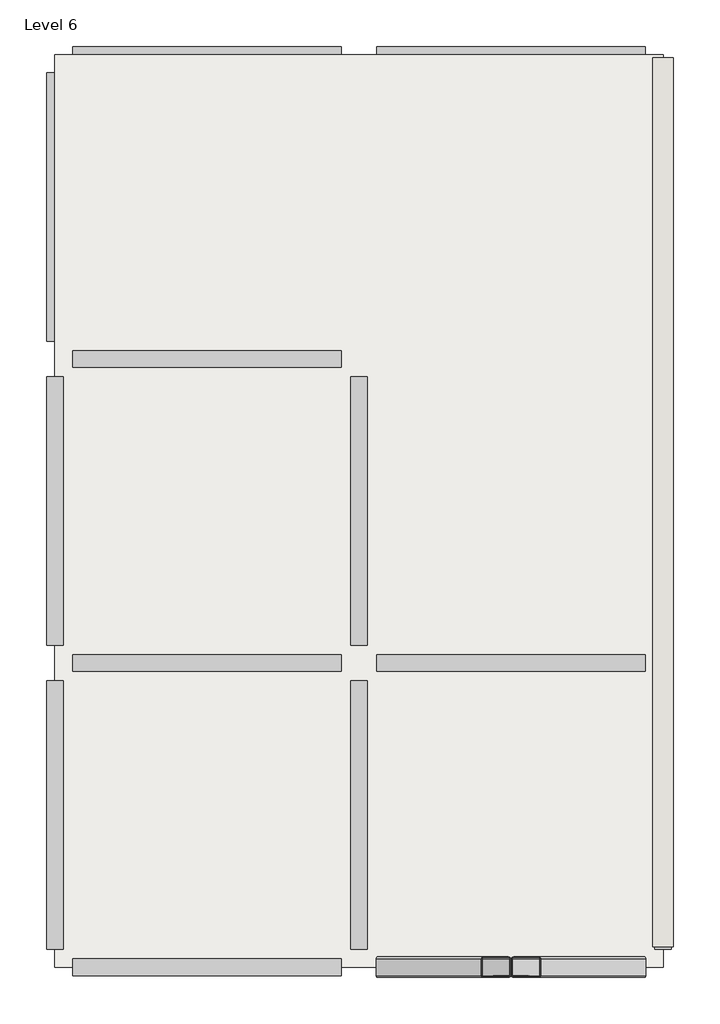
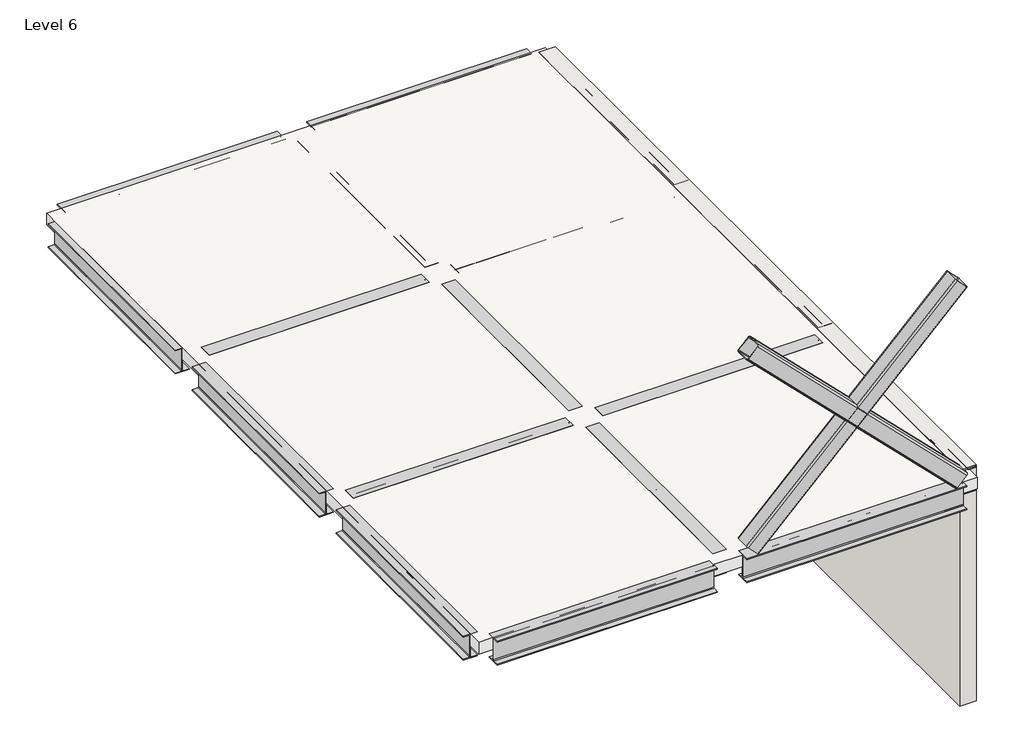
# One storey: 17 beams, 2 members, 1 slab, 1 wall.
"""IFC4 building model written with IfcOpenShell, lengths in millimetres."""

from ifc_helpers import new_model, si_unit, frame, origin, place, context, project, spatial, polyline, outline, extrude, transform, mapped, element, save
from components import ub_universal_beams_ub305x165x40_60ab2ee1, m_hss_square_hss203_2x203_2x9_5_07d005dd

model = new_model("IFC4")

# Units and contexts
model_context = context("Model", 3, world=origin())
ifc_project = project(units=[si_unit("LENGTHUNIT", "METRE", prefix="MILLI")], contexts=[model_context])

# Site, building, storey
site = spatial("IfcSite", under=ifc_project)
building = spatial("IfcBuilding", under=site)
storey = spatial("IfcBuildingStorey", under=building, Name="Level 6", Elevation=15000.0)

# Beams
placement = place(None, origin())
ub_universal_beams_ub305x165x40_shape = ub_universal_beams_ub305x165x40_60ab2ee1(model_context)
element("IfcBeam", 1, ObjectType="UB-Universal Beams : UB305x165x40", at=placement, inside=storey, context=model_context, shape_type="MappedRepresentation", body=[
    mapped(ub_universal_beams_ub305x165x40_shape, transform((18435.1404262, -6314.7314166, 14848.3), x_axis=(-1.0, 0.0, 0.0), y_axis=(0.0, -1.0, 0.0), z_axis=(0.0, 0.0, 1.0))),
])
element("IfcBeam", 2, ObjectType="UB-Universal Beams : UB305x165x40", at=placement, inside=storey, context=model_context, shape_type="MappedRepresentation", body=[
    mapped(ub_universal_beams_ub305x165x40_shape, transform((15435.1404262, -6314.7314166, 14848.3), x_axis=(-1.0, 0.0, 0.0), y_axis=(0.0, -1.0, 0.0), z_axis=(0.0, 0.0, 1.0))),
])
element("IfcBeam", 3, ObjectType="UB-Universal Beams : UB305x165x40", at=placement, inside=storey, context=model_context, shape_type="MappedRepresentation", body=[
    mapped(ub_universal_beams_ub305x165x40_shape, transform((13935.1404262, -4814.7314166, 14848.3), x_axis=(0.0, 1.0, 0.0), y_axis=(-1.0, 0.0, 0.0), z_axis=(0.0, 0.0, 1.0))),
])
element("IfcBeam", 4, ObjectType="UB-Universal Beams : UB305x165x40", at=placement, inside=storey, context=model_context, shape_type="MappedRepresentation", body=[
    mapped(ub_universal_beams_ub305x165x40_shape, transform((13935.1404262, -1814.7314166, 14848.3), x_axis=(0.0, 1.0, 0.0), y_axis=(-1.0, 0.0, 0.0), z_axis=(0.0, 0.0, 1.0))),
])
element("IfcBeam", 5, ObjectType="UB-Universal Beams : UB305x165x40", at=placement, inside=storey, context=model_context, shape_type="MappedRepresentation", body=[
    mapped(ub_universal_beams_ub305x165x40_shape, transform((13935.1404262, 1185.2685834, 14848.3), x_axis=(0.0, 1.0, 0.0), y_axis=(-1.0, 0.0, 0.0), z_axis=(0.0, 0.0, 1.0))),
])
element("IfcBeam", 6, ObjectType="UB-Universal Beams : UB305x165x40", at=placement, inside=storey, context=model_context, shape_type="MappedRepresentation", body=[
    mapped(ub_universal_beams_ub305x165x40_shape, transform((18435.1404262, -3314.7314166, 14848.3), x_axis=(-1.0, 0.0, 0.0), y_axis=(0.0, -1.0, 0.0), z_axis=(0.0, 0.0, 1.0))),
])
element("IfcBeam", 7, ObjectType="UB-Universal Beams : UB305x165x40", at=placement, inside=storey, context=model_context, shape_type="MappedRepresentation", body=[
    mapped(ub_universal_beams_ub305x165x40_shape, transform((15435.1404262, -3314.7314166, 14848.3), x_axis=(-1.0, 0.0, 0.0), y_axis=(0.0, -1.0, 0.0), z_axis=(0.0, 0.0, 1.0))),
])
element("IfcBeam", 8, ObjectType="UB-Universal Beams : UB305x165x40", at=placement, inside=storey, context=model_context, shape_type="MappedRepresentation", body=[
    mapped(ub_universal_beams_ub305x165x40_shape, transform((18435.1404262, -314.7314166, 14848.3), x_axis=(-1.0, 0.0, 0.0), y_axis=(0.0, -1.0, 0.0), z_axis=(0.0, 0.0, 1.0))),
])
element("IfcBeam", 9, ObjectType="UB-Universal Beams : UB305x165x40", at=placement, inside=storey, context=model_context, shape_type="MappedRepresentation", body=[
    mapped(ub_universal_beams_ub305x165x40_shape, transform((15435.1404262, -314.7314166, 14848.3), x_axis=(-1.0, 0.0, 0.0), y_axis=(0.0, -1.0, 0.0), z_axis=(0.0, 0.0, 1.0))),
])
element("IfcBeam", 10, ObjectType="UB-Universal Beams : UB305x165x40", at=placement, inside=storey, context=model_context, shape_type="MappedRepresentation", body=[
    mapped(ub_universal_beams_ub305x165x40_shape, transform((18435.1404262, 2685.2685834, 14848.3), x_axis=(-1.0, 0.0, 0.0), y_axis=(0.0, -1.0, 0.0), z_axis=(0.0, 0.0, 1.0))),
])
element("IfcBeam", 11, ObjectType="UB-Universal Beams : UB305x165x40", at=placement, inside=storey, context=model_context, shape_type="MappedRepresentation", body=[
    mapped(ub_universal_beams_ub305x165x40_shape, transform((15435.1404262, 2685.2685834, 14848.3), x_axis=(-1.0, 0.0, 0.0), y_axis=(0.0, -1.0, 0.0), z_axis=(0.0, 0.0, 1.0))),
])
element("IfcBeam", 12, ObjectType="UB-Universal Beams : UB305x165x40", at=placement, inside=storey, context=model_context, shape_type="MappedRepresentation", body=[
    mapped(ub_universal_beams_ub305x165x40_shape, transform((16935.1404262, -4814.7314166, 14848.3), x_axis=(0.0, 1.0, 0.0), y_axis=(-1.0, 0.0, 0.0), z_axis=(0.0, 0.0, 1.0))),
])
element("IfcBeam", 13, ObjectType="UB-Universal Beams : UB305x165x40", at=placement, inside=storey, context=model_context, shape_type="MappedRepresentation", body=[
    mapped(ub_universal_beams_ub305x165x40_shape, transform((16935.1404262, -1814.7314166, 14848.3), x_axis=(0.0, 1.0, 0.0), y_axis=(-1.0, 0.0, 0.0), z_axis=(0.0, 0.0, 1.0))),
])
element("IfcBeam", 14, ObjectType="UB-Universal Beams : UB305x165x40", at=placement, inside=storey, context=model_context, shape_type="MappedRepresentation", body=[
    mapped(ub_universal_beams_ub305x165x40_shape, transform((16935.1404262, 1185.2685834, 14848.3), x_axis=(0.0, 1.0, 0.0), y_axis=(-1.0, 0.0, 0.0), z_axis=(0.0, 0.0, 1.0))),
])
element("IfcBeam", 15, ObjectType="UB-Universal Beams : UB305x165x40", at=placement, inside=storey, context=model_context, shape_type="MappedRepresentation", body=[
    mapped(ub_universal_beams_ub305x165x40_shape, transform((19935.1404262, -1814.7314166, 14848.3), x_axis=(0.0, 1.0, 0.0), y_axis=(-1.0, 0.0, 0.0), z_axis=(0.0, 0.0, 1.0))),
])
element("IfcBeam", 16, ObjectType="UB-Universal Beams : UB305x165x40", at=placement, inside=storey, context=model_context, shape_type="MappedRepresentation", body=[
    mapped(ub_universal_beams_ub305x165x40_shape, transform((19935.1404262, 1185.2685834, 14848.3), x_axis=(0.0, 1.0, 0.0), y_axis=(-1.0, 0.0, 0.0), z_axis=(0.0, 0.0, 1.0))),
])
element("IfcBeam", 17, ObjectType="UB-Universal Beams : beam", at=placement, inside=storey, context=model_context, shape_type="MappedRepresentation", body=[
    mapped(ub_universal_beams_ub305x165x40_shape, transform((19935.1404262, -4814.7314166, 14848.3), x_axis=(0.0, 1.0, 0.0), y_axis=(-1.0, 0.0, 0.0), z_axis=(0.0, 0.0, 1.0))),
])

# Members
m_hss_square_hss203_2x203_2x9_5_shape = m_hss_square_hss203_2x203_2x9_5_07d005dd(model_context)
element("IfcMember", 18, ObjectType="M_HSS Square : HSS203.2X203.2X9.5", at=placement, inside=storey, context=model_context, shape_type="MappedRepresentation", body=[
    mapped(m_hss_square_hss203_2x203_2x9_5_shape, transform((18435.1404262, -6314.7314166, 16348.3), x_axis=(-0.7071067811865478, 0.0, 0.7071067811865476), y_axis=(0.0, -1.0000000000000002, 0.0), z_axis=(0.7071067811865476, 0.0, 0.7071067811865478))),
])
element("IfcMember", 19, ObjectType="M_HSS Square : HSS203.2X203.2X9.5", at=placement, inside=storey, context=model_context, shape_type="MappedRepresentation", body=[
    mapped(m_hss_square_hss203_2x203_2x9_5_shape, transform((18435.1404262, -6314.7314166, 16348.3), x_axis=(-0.7071067811865478, 0.0, -0.7071067811865475), y_axis=(0.0, -1.0000000000000002, 0.0), z_axis=(-0.7071067811865475, 0.0, 0.7071067811865478))),
])

# Slab
element("IfcSlab", 20, ObjectType="150mm Foundation Slab", at=placement, inside=storey, context=model_context, shape_type="SweptSolid", body=[
    extrude(outline(polyline([(13935.1404262, -6314.7314166), (13935.1404262, 2685.2685834), (19935.1404262, 2685.2685834), (19935.1404262, -6314.7314166), (13935.1404262, -6314.7314166)])), frame((0.0, 0.0, 14850.0), z_axis=(0.0, 0.0, 1.0), x_axis=(1.0, 0.0, 0.0)), (0.0, 0.0, 1.0), 150.0),
])

# Wall
element("IfcWall", 21, ObjectType="Generic - 200mm", at=placement, inside=storey, context=model_context, shape_type="SweptSolid", body=[
    extrude(outline(polyline([(19835.1404262, -6114.7314166), (19835.1404262, 2655.9792615), (20035.1404262, 2655.9792615), (20035.1404262, -6114.7314166), (19835.1404262, -6114.7314166)])), frame((0.0, 0.0, 12000.0), z_axis=(0.0, 0.0, 1.0), x_axis=(1.0, 0.0, 0.0)), (0.0, 0.0, 1.0), 3000.0),
])

save(model, "model.ifc")

# Revit data of these elements
# Type "UB-Universal Beams : UB305x165x40"
#   Section Name Key = "UB305X165X40"
#   Width = 16.5 cm
#   Web Thickness = 0.6 cm
#   Web Fillet = 0.89 cm
#   Warping Constant = 164000.0 cm⁶
#   Torsional Moment of Inertia = 14.70 cm⁴
#   Section Area = 51.3 cm²
#   Plastic Modulus weak axis = 142.0 cm³
#   Plastic Modulus strong axis = 623.0 cm³
#   Nominal Weight = 40.2999 kgf/m
#   Moment of Inertia weak axis = 764.00 cm⁴
#   Moment of Inertia strong axis = 8503.00 cm⁴
#   Height = 30.34 cm
#   Flange Thickness = 1.02 cm
#   Elastic Modulus weak axis = 92.6 cm³
#   Elastic Modulus strong axis = 560.0 cm³
#   Centroid Vertical = 15.17 cm
#   Centroid Horizontal = 8.25 cm
#   Bolt Spacing = 9.0 cm
#   Length [instance default] = 1.5 m
#   Structural Material [instance default] = Metal - Steel 43-275
#   Type Comments = ""
#   Assembly Code = ""
# Type "UB-Universal Beams : beam"
#   Section Name Key = "UB305X165X40"
#   Width = 16.5 cm
#   Web Thickness = 0.6 cm
#   Web Fillet = 0.89 cm
#   Warping Constant = 164000.0 cm⁶
#   Torsional Moment of Inertia = 14.70 cm⁴
#   Section Area = 51.3 cm²
#   Plastic Modulus weak axis = 142.0 cm³
#   Plastic Modulus strong axis = 623.0 cm³
#   Nominal Weight = 40.2999 kgf/m
#   Moment of Inertia weak axis = 764.00 cm⁴
#   Moment of Inertia strong axis = 8503.00 cm⁴
#   Height = 30.34 cm
#   Flange Thickness = 1.02 cm
#   Elastic Modulus weak axis = 92.6 cm³
#   Elastic Modulus strong axis = 560.0 cm³
#   Centroid Vertical = 15.17 cm
#   Centroid Horizontal = 8.25 cm
#   Bolt Spacing = 9.0 cm
#   Length [instance default] = 1.5 m
#   Structural Material [instance default] = Metal - Steel 43-275
#   Type Comments = ""
#   Assembly Code = ""
# Type "M_HSS Square : HSS203.2X203.2X9.5"
#   Section Name Key = "HSS 8X8X3/8"
#   Width = 20.3 cm
#   Wall Nominal Thickness = 0.953 cm
#   Wall Design Thickness = 0.886 cm
#   Torsional Moment of Inertia = 6660.00 cm⁴
#   Torsional Modulus = 10930171.7 cm³
#   Section Area = 67.1 cm²
#   Plastic Modulus weak axis = 482.0 cm³
#   Plastic Modulus strong axis = 482.0 cm³
#   Outer Fillet = 1.906 cm
#   Nominal Weight = 55.9998 kgf/m
#   Moment of Inertia weak axis = 4160.00 cm⁴
#   Moment of Inertia strong axis = 4160.00 cm⁴
#   Length [instance default] = 1.524 m
#   Inner Fillet = 0.953 cm
#   Height = 20.3 cm
#   Elastic Modulus weak axis = 408.0 cm³
#   Elastic Modulus strong axis = 408.0 cm³
#   Centroid Vertical = 10.15 cm
#   Centroid Horizontal = 10.15 cm
#   Structural Material [instance default] = Steel, 45-345
# Type "150mm Foundation Slab"
#   Layers, outside or top first: 0.15 m "Concrete, Cast-in-Place gray" (function 1)
# Type "Generic - 200mm"
#   Layers, outside or top first: 0.2 m no material (function 1)
# Elements 1, 2, 3, 4, 5, 6, 7, 8, 9, 10, 11, 12, 13, 14, 15, 16 (IfcBeam, "UB-Universal Beams : UB305x165x40")
#   Structural Material = Metal - Steel 43-275
#   Phase Created = New Construction
#   Materials on its faces: "Metal - Steel 43-275"
# Element 17 (IfcBeam, "UB-Universal Beams : beam")
#   Structural Material = Metal - Steel 43-275
#   Phase Created = New Construction
#   Materials on its faces: "Metal - Steel 43-275"
# Elements 18, 19 (IfcMember, "M_HSS Square : HSS203.2X203.2X9.5")
#   Comments = ""
#   Structural Material = Metal - Steel 43-275
#   Phase Created = New Construction
#   Materials on its faces: "Metal - Steel 43-275"
# Element 20 (IfcSlab, "150mm Foundation Slab")
#   built-in parameter 1001955 = 3.14159 (stored number, unit not read)
#   Height Offset From Level = 0 m
#   built-in parameter 1001954 = 1
#   Phase Created = New Construction
#   Materials on its faces: "Concrete, Cast-in-Place gray"
# Element 21 (IfcWall, "Generic - 200mm")
#   Comments = ""
#   built-in parameter 1001111 = -3 m
#   Top Offset = 0 m
#   Base Offset = -3 m
#   wall height = 3 m
#   Phase Created = New Construction
#   Base Constraint = Level 6
#   Top Constraint = Level 6
#   Materials on its faces: "Default Wall"
# Materials
#   "Metal - Steel 43-275": class "Metal", colour RGB 247 247 247, transparency 0, Cost = 0
#   "Steel, 45-345": class "Metal", colour RGB 247 247 247, transparency 0, Description = "Steel 345 MPa", Cost = 0
#   "Concrete, Cast-in-Place gray": class "Concrete", colour RGB 192 192 192, transparency 0, Description = "Cast-in-place concrete", Cost = 0
#   "Default Wall": colour RGB 128 128 128, transparency 0, Cost = 0
